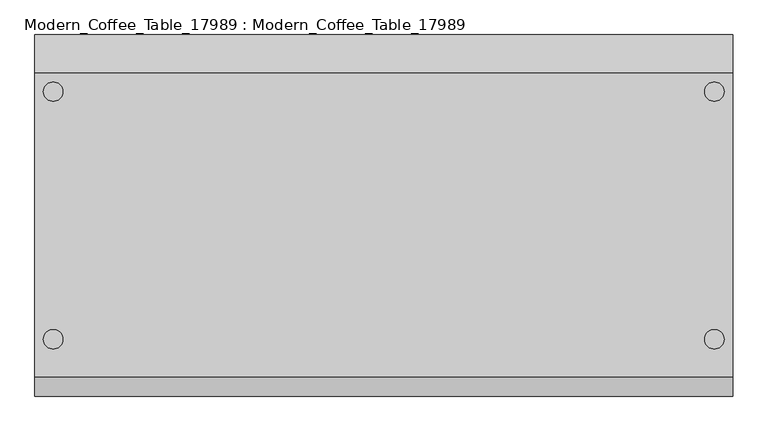
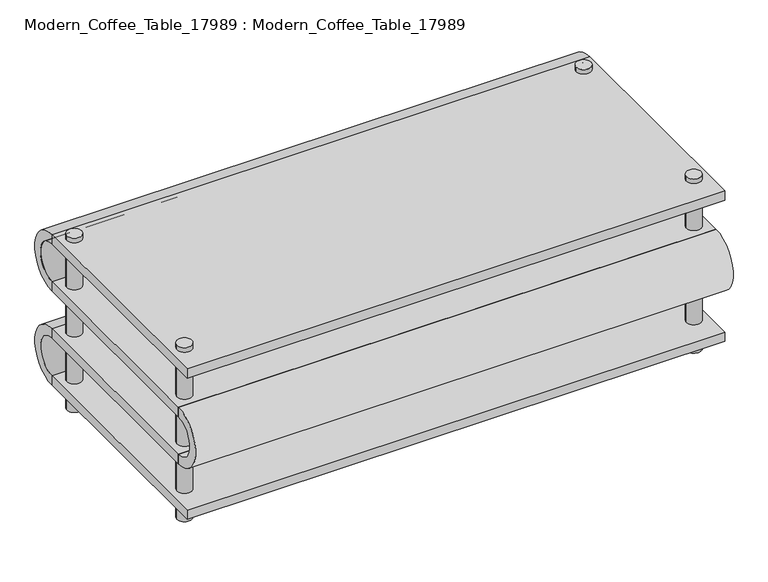
"""IFC4 building model written with IfcOpenShell, lengths in millimetres: proxy geometry, Modern_Coffee_Table_17989 : Modern_Coffee_Table_17989."""

from ifc_helpers import new_model, si_unit, point, frame, frame_2d, origin, origin_with_axes, place, context, project, spatial, polyline, circle_curve, trimmed, segment, composite_curve, outline, extrude, source, transform, mapped, element, save


def modern_coffee_table_17989_modern_coffee_table_17989_d3a860c8(model_context):
    return source(origin(), model_context, "Body", "SweptSolid", [
        extrude(outline(polyline([(457.2, -76.2), (457.2, -673.1), (-914.4, -673.1), (-914.4, -76.2), (457.2, -76.2)])), frame((0.0, 0.0, 431.8), z_axis=(0.0, 0.0, 1.0), x_axis=(1.0, 0.0, 0.0)), (0.0, 0.0, 1.0), 25.4),
        extrude(outline(polyline([(457.2, -76.2), (457.2, -673.1), (-914.4, -673.1), (-914.4, -76.2), (457.2, -76.2)])), frame((0.0, 0.0, 50.8), z_axis=(0.0, 0.0, 1.0), x_axis=(1.0, 0.0, 0.0)), (0.0, 0.0, 1.0), 25.4),
        extrude(outline(polyline([(457.2, -76.2), (457.2, -635.0), (-914.4, -635.0), (-914.4, -76.2), (457.2, -76.2)])), frame((0.0, 0.0, 304.8), z_axis=(0.0, 0.0, 1.0), x_axis=(1.0, 0.0, 0.0)), (0.0, 0.0, 1.0), 25.4),
        extrude(outline(polyline([(457.2, -76.2), (457.2, -635.0), (-914.4, -635.0), (-914.4, -76.2), (457.2, -76.2)])), frame((0.0, 0.0, 177.8), z_axis=(0.0, 0.0, 1.0), x_axis=(1.0, 0.0, 0.0)), (0.0, 0.0, 1.0), 25.4),
        extrude(outline(composite_curve([segment(trimmed(circle_curve(frame_2d((-76.2, 381.0)), 50.8), [point((-76.2, 330.2))], [point((-76.2, 431.8))], True, "CARTESIAN"), True, "CONTINUOUS"), segment(polyline([(-76.2, 431.8), (-76.2, 457.2)]), True, "CONTINUOUS"), segment(trimmed(circle_curve(frame_2d((-76.2, 381.0)), 76.2), [point((-76.2, 457.2))], [point((-76.2, 304.8))], False, "CARTESIAN"), True, "CONTINUOUS"), segment(polyline([(-76.2, 304.8), (-76.2, 330.2)]), True, "CONTINUOUS")], self_intersect=False)), frame((-914.4, 0.0, 0.0), z_axis=(1.0, 0.0, 0.0), x_axis=(0.0, 1.0, 0.0)), (0.0, 0.0, 1.0), 1371.6),
        extrude(outline(composite_curve([segment(polyline([(-635.0, 203.2), (-635.0, 177.8)]), True, "CONTINUOUS"), segment(trimmed(circle_curve(frame_2d((-635.0, 254.0)), 76.2), [point((-635.0, 177.8))], [point((-635.0, 330.2))], False, "CARTESIAN"), True, "CONTINUOUS"), segment(polyline([(-635.0, 330.2), (-635.0, 304.8)]), True, "CONTINUOUS"), segment(trimmed(circle_curve(frame_2d((-635.0, 254.0)), 50.8), [point((-635.0, 304.8))], [point((-635.0, 203.2))], True, "CARTESIAN"), True, "CONTINUOUS")], self_intersect=False)), frame((-914.4, 0.0, 0.0), z_axis=(1.0, 0.0, 0.0), x_axis=(0.0, 1.0, 0.0)), (0.0, 0.0, 1.0), 1371.6),
        extrude(outline(composite_curve([segment(trimmed(circle_curve(frame_2d((-76.2, 127.0)), 50.8), [point((-76.2, 76.2))], [point((-76.2, 177.8))], True, "CARTESIAN"), True, "CONTINUOUS"), segment(polyline([(-76.2, 177.8), (-76.2, 203.2)]), True, "CONTINUOUS"), segment(trimmed(circle_curve(frame_2d((-76.2, 127.0)), 76.2), [point((-76.2, 203.2))], [point((-76.2, 50.8))], False, "CARTESIAN"), True, "CONTINUOUS"), segment(polyline([(-76.2, 50.8), (-76.2, 76.2)]), True, "CONTINUOUS")], self_intersect=False)), frame((-914.4, 0.0, 0.0), z_axis=(1.0, 0.0, 0.0), x_axis=(0.0, 1.0, 0.0)), (0.0, 0.0, 1.0), 1371.6),
        extrude(outline(composite_curve([segment(trimmed(circle_curve(frame_2d((-878.4789755, -112.1210245)), 19.05), [point((-897.5289755, -112.1210245))], [point((-859.4289755, -112.1210245))], False, "CARTESIAN"), True, "CONTINUOUS"), segment(trimmed(circle_curve(frame_2d((-878.4789755, -112.1210245)), 19.05), [point((-859.4289755, -112.1210245))], [point((-897.5289755, -112.1210245))], False, "CARTESIAN"), True, "CONTINUOUS")], self_intersect=False)), origin_with_axes(), (0.0, 0.0, 1.0), 469.9),
        extrude(outline(composite_curve([segment(trimmed(circle_curve(frame_2d((-878.4789755, -599.0789755)), 19.05), [point((-897.5289755, -599.0789755))], [point((-859.4289755, -599.0789755))], False, "CARTESIAN"), True, "CONTINUOUS"), segment(trimmed(circle_curve(frame_2d((-878.4789755, -599.0789755)), 19.05), [point((-859.4289755, -599.0789755))], [point((-897.5289755, -599.0789755))], False, "CARTESIAN"), True, "CONTINUOUS")], self_intersect=False)), origin_with_axes(), (0.0, 0.0, 1.0), 469.9),
        extrude(outline(composite_curve([segment(trimmed(circle_curve(frame_2d((421.2789755, -599.0789755)), 19.05), [point((402.2289755, -599.0789755))], [point((440.3289755, -599.0789755))], False, "CARTESIAN"), True, "CONTINUOUS"), segment(trimmed(circle_curve(frame_2d((421.2789755, -599.0789755)), 19.05), [point((440.3289755, -599.0789755))], [point((402.2289755, -599.0789755))], False, "CARTESIAN"), True, "CONTINUOUS")], self_intersect=False)), origin_with_axes(), (0.0, 0.0, 1.0), 469.9),
        extrude(outline(composite_curve([segment(trimmed(circle_curve(frame_2d((421.2789755, -112.1210245)), 19.05), [point((402.2289755, -112.1210245))], [point((440.3289755, -112.1210245))], False, "CARTESIAN"), True, "CONTINUOUS"), segment(trimmed(circle_curve(frame_2d((421.2789755, -112.1210245)), 19.05), [point((440.3289755, -112.1210245))], [point((402.2289755, -112.1210245))], False, "CARTESIAN"), True, "CONTINUOUS")], self_intersect=False)), origin_with_axes(), (0.0, 0.0, 1.0), 469.9),
    ])


if __name__ == "__main__":
    model = new_model("IFC4")
    model_context = context("Model", 3, world=origin())
    ifc_project = project(units=[si_unit("LENGTHUNIT", "METRE", prefix="MILLI")], contexts=[model_context])
    site = spatial("IfcSite", under=ifc_project)
    building = spatial("IfcBuilding", under=site)
    placement = place(None, origin())
    modern_coffee_table_17989_modern_coffee_table_17989_shape = modern_coffee_table_17989_modern_coffee_table_17989_d3a860c8(model_context)
    element("IfcBuildingElementProxy", 1, Name="Modern_Coffee_Table_17989 : Modern_Coffee_Table_17989", ObjectType="Modern_Coffee_Table_17989 : Modern_Coffee_Table_17989", at=placement, inside=building, context=model_context, shape_type="MappedRepresentation", body=[
        mapped(modern_coffee_table_17989_modern_coffee_table_17989_shape, transform((0.0, 0.0, 0.0), x_axis=(1.0, 0.0, 0.0), y_axis=(0.0, 1.0, 0.0), z_axis=(0.0, 0.0, 1.0))),
    ])
    save(model, "model.ifc")

# Revit data of these elements
# Type "Modern_Coffee_Table_17989 : Modern_Coffee_Table_17989"
#   Default Elevation = 0
# Element 1 (IfcBuildingElementProxy, "Modern_Coffee_Table_17989 : Modern_Coffee_Table_17989")
#   Materials on its faces: "1 Wood", "1 Glass", "1 Metal"
# Materials
#   "1 Wood": class "Glass", colour RGB 81 52 39, transparency 0, Cost = 0
#   "1 Glass": class "Glass", colour RGB 236 240 239, transparency 0.85, Cost = 0
#   "1 Metal": class "Glass", colour RGB 244 244 244, transparency 0, Cost = 0
